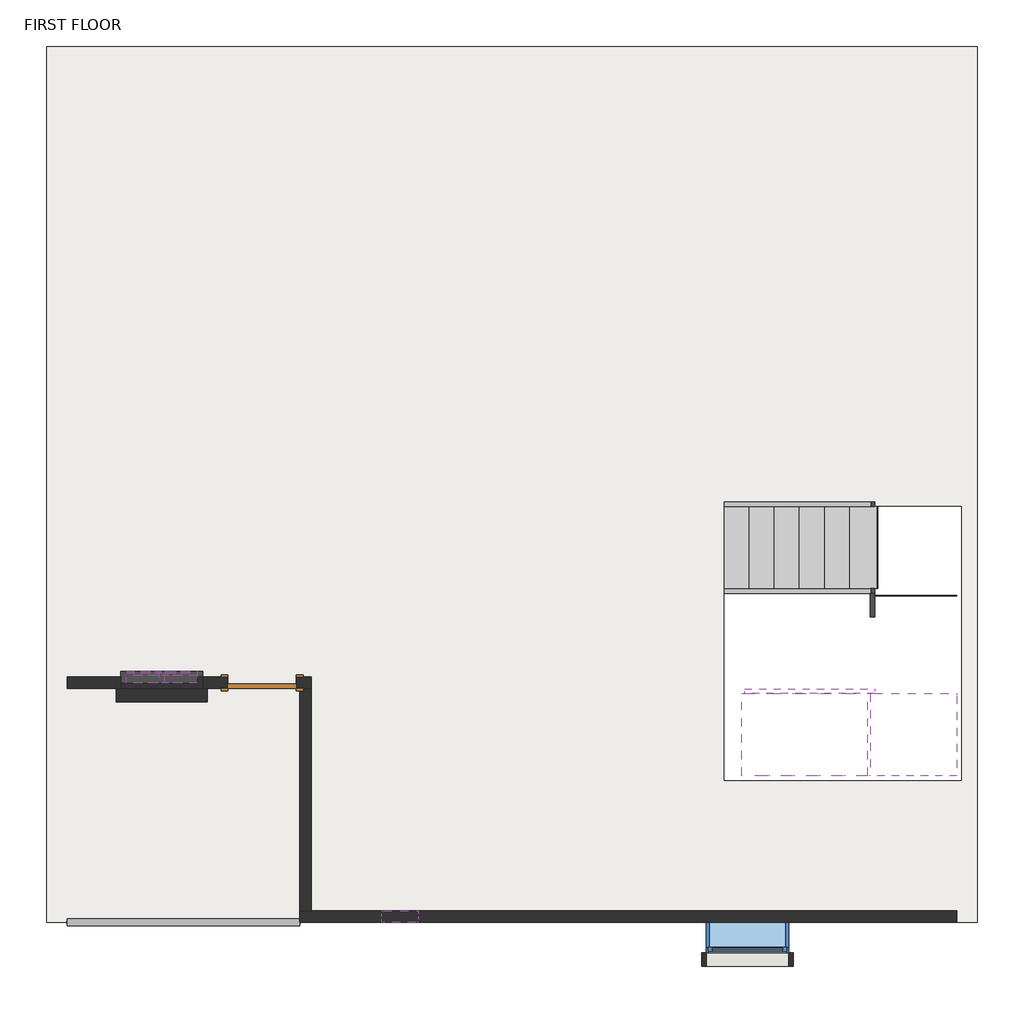
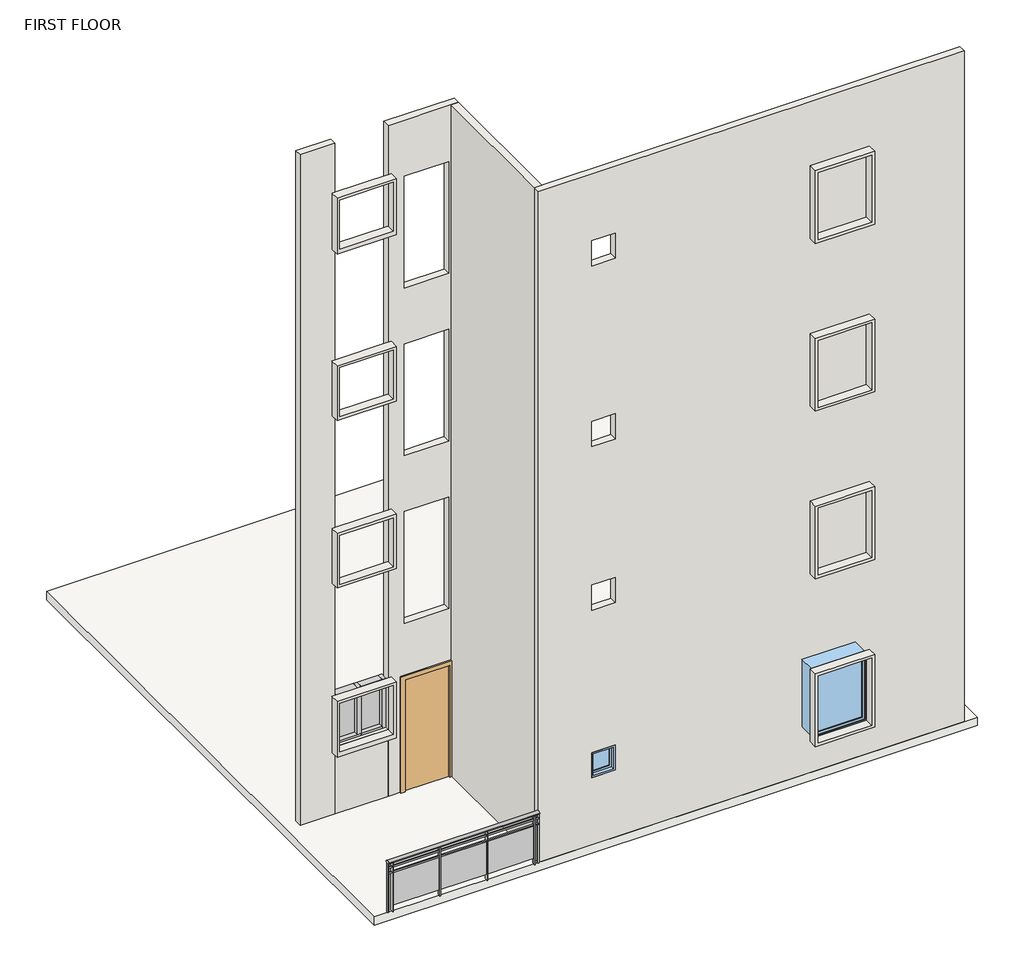
# One storey, incomplete: 15 members, 7 walls, 3 plates, 3 stair flights, 2 slabs, 2 windows, 1 door, 1 railing.
"""IFC4 building model written with IfcOpenShell, lengths in millimetres."""

from ifc_helpers import new_model, si_unit, point, frame, origin, place, context, project, spatial, polyline, ellipse_curve, trimmed, outline, extrude, faceted_brep, transform, mapped, element, save
from ifc_brep_helpers import plane_surface, extruded_surface, advanced_brep
from components import door_e00f436c, member_429f6687, member_d959a85f, member_843225dc, member_54f829b7, system_panel_glazed_1e360deb, system_panel_glazed_8fc33089, non_monolithic_landing_440175ab, stair_flight_60bc6d16, stair_flight_15cb6ebf, stair_flight_16b82674, walls_8_walls_8_31a24d2c, walls_9_walls_9_93cd2fbd, fixed_bw_be0fa6e9, fixed_ven_0bde2124

model = new_model("IFC4")

# Units and contexts
model_context = context("Model", 3, world=origin())
ifc_project = project(units=[si_unit("LENGTHUNIT", "METRE", prefix="MILLI")], contexts=[model_context])

# Site, building, storey
site = spatial("IfcSite", under=ifc_project)
building = spatial("IfcBuilding", under=site)
storey = spatial("IfcBuildingStorey", under=building, Name="FIRST FLOOR", Elevation=3048.0)

# Door
placement = place(None, origin())
door_shape = door_e00f436c(model_context)
element("IfcDoor", 1, ObjectType="Single-Flush : 36\" x 84\"", at=placement, inside=storey, context=model_context, shape_type="MappedRepresentation", body=[
    mapped(door_shape, transform((-4124.5569651, 3118.5055142, 3048.0), x_axis=(1.0, 0.0, 0.0), y_axis=(0.0, 1.0, 0.0), z_axis=(0.0, 0.0, 1.0))),
])

# Members
member_shape = member_429f6687(model_context)
element("IfcMember", 2, ObjectType="Rectangular Mullion : 2.5\" x 5\" rectangular", at=placement, inside=storey, context=model_context, shape_type="MappedRepresentation", body=[
    mapped(member_shape, transform((-4848.4569651, 3182.0055142, 5156.2), x_axis=(0.0, 0.0, 1.0), y_axis=(0.0, -1.0, 0.0), z_axis=(1.0, 0.0, 0.0))),
])
element("IfcMember", 3, ObjectType="Rectangular Mullion : 2.5\" x 5\" rectangular", at=placement, inside=storey, context=model_context, shape_type="MappedRepresentation", body=[
    mapped(member_shape, transform((-5635.8569651, 3182.0055142, 4237.4584417), x_axis=(0.0, 0.0, -1.0), y_axis=(0.0, -1.0, 0.0), z_axis=(-1.0, 0.0, 0.0))),
])
member_2_shape = member_d959a85f(model_context)
element("IfcMember", 4, ObjectType="Rectangular Mullion : 2.5\" x 5\" rectangular", at=placement, inside=storey, context=model_context, shape_type="MappedRepresentation", body=[
    mapped(member_2_shape, transform((-4784.9569651, 3182.0055142, 4237.4584417), x_axis=(1.0, 0.0, 0.0), y_axis=(0.0, -1.0, 0.0), z_axis=(0.0, 0.0, -1.0))),
])
element("IfcMember", 5, ObjectType="Rectangular Mullion : 2.5\" x 5\" rectangular", at=placement, inside=storey, context=model_context, shape_type="MappedRepresentation", body=[
    mapped(member_2_shape, transform((-4784.9569651, 3182.0055142, 4237.4584417), x_axis=(1.0, 0.0, 0.0), y_axis=(0.0, -1.0, 0.0), z_axis=(0.0, 0.0, -1.0))),
])
element("IfcMember", 6, ObjectType="Rectangular Mullion : 2.5\" x 5\" rectangular", at=placement, inside=storey, context=model_context, shape_type="MappedRepresentation", body=[
    mapped(member_2_shape, transform((-5699.3569651, 3182.0055142, 5156.2), x_axis=(-1.0, 0.0, 0.0), y_axis=(0.0, -1.0, 0.0), z_axis=(0.0, 0.0, 1.0))),
])
element("IfcMember", 7, ObjectType="Rectangular Mullion : 2.5\" x 5\" rectangular", at=placement, inside=storey, context=model_context, shape_type="MappedRepresentation", body=[
    mapped(member_2_shape, transform((-5699.3569651, 3182.0055142, 5156.2), x_axis=(-1.0, 0.0, 0.0), y_axis=(0.0, -1.0, 0.0), z_axis=(0.0, 0.0, 1.0))),
])
member_3_shape = member_843225dc(model_context)
element("IfcMember", 8, ObjectType="Rectangular Mullion : 2.5\" x 5\" rectangular", at=placement, inside=storey, context=model_context, shape_type="MappedRepresentation", body=[
    mapped(member_3_shape, transform((-4848.4569651, 3182.0055142, 5156.2), x_axis=(0.0, 0.0, 1.0), y_axis=(0.0, -1.0, 0.0), z_axis=(1.0, 0.0, 0.0))),
])
element("IfcMember", 9, ObjectType="Rectangular Mullion : 2.5\" x 5\" rectangular", at=placement, inside=storey, context=model_context, shape_type="MappedRepresentation", body=[
    mapped(member_3_shape, transform((-5273.9069651, 3182.0055142, 5156.2), x_axis=(0.0, 0.0, 1.0), y_axis=(0.0, -1.0, 0.0), z_axis=(1.0, 0.0, 0.0))),
])
element("IfcMember", 10, ObjectType="Rectangular Mullion : 2.5\" x 5\" rectangular", at=placement, inside=storey, context=model_context, shape_type="MappedRepresentation", body=[
    mapped(member_3_shape, transform((-5635.8569651, 3182.0055142, 4237.4584417), x_axis=(0.0, 0.0, -1.0), y_axis=(0.0, -1.0, 0.0), z_axis=(-1.0, 0.0, 0.0))),
])
element("IfcMember", 11, ObjectType="Rectangular Mullion : 2.5\" x 5\" rectangular", at=placement, inside=storey, context=model_context, shape_type="MappedRepresentation", body=[
    mapped(member_3_shape, transform((-5210.4069651, 3182.0055142, 4237.4584417), x_axis=(0.0, 0.0, -1.0), y_axis=(0.0, -1.0, 0.0), z_axis=(-1.0, 0.0, 0.0))),
])
member_4_shape = member_54f829b7(model_context)
element("IfcMember", 12, ObjectType="Rectangular Mullion : 2.5\" x 5\" rectangular", at=placement, inside=storey, context=model_context, shape_type="MappedRepresentation", body=[
    mapped(member_4_shape, transform((-5242.1569651, 3182.0055142, 4237.4584417), x_axis=(1.0, 0.0, 0.0), y_axis=(0.0, -1.0, 0.0), z_axis=(0.0, 0.0, -1.0))),
])
element("IfcMember", 13, ObjectType="Stringer - 2\" Width", at=placement, inside=storey, context=model_context, shape_type="SweptSolid", body=[
    extrude(outline(polyline([(3260.114512, 1018.9430349), (3048.0, 1018.9430349), (3048.0, 1257.0285467), (3919.7057504, 2695.3430349), (4276.114512, 2695.3430349), (3260.114512, 1018.9430349)])), frame((0.0, 5080.6555142, 0.0), z_axis=(0.0, 1.0, 0.0), x_axis=(0.0, 0.0, 1.0)), (0.0, 0.0, 1.0), 50.8),
])
element("IfcMember", 14, ObjectType="Stringer - 2\" Width", at=placement, inside=storey, context=model_context, shape_type="SweptSolid", body=[
    extrude(outline(polyline([(3260.114512, 1018.9430349), (3048.0, 1018.9430349), (3048.0, 1257.0285467), (3919.7057504, 2695.3430349), (4276.114512, 2695.3430349), (3260.114512, 1018.9430349)])), frame((0.0, 4115.4555142, 0.0), z_axis=(0.0, 1.0, 0.0), x_axis=(0.0, 0.0, 1.0)), (0.0, 0.0, 1.0), 50.8),
])
element("IfcMember", 15, ObjectType="Stringer - 2\" Width", at=placement, inside=storey, context=model_context, shape_type="SweptSolid", body=[
    extrude(outline(polyline([(4115.4555142, 4445.4478453), (4115.4555142, 4089.0390838), (3048.6555142, 4735.5845383), (3048.6555142, 5091.9932998), (4115.4555142, 4445.4478453)])), frame((2644.5430349, 0.0, 0.0), z_axis=(1.0, 0.0, 0.0), x_axis=(0.0, 1.0, 0.0)), (0.0, 0.0, 1.0), 50.8),
])
element("IfcMember", 16, ObjectType="Stringer - 2\" Width", at=placement, inside=storey, context=model_context, shape_type="SweptSolid", body=[
    extrude(outline(polyline([(4904.9178717, 2695.3430349), (5261.3266332, 2695.3430349), (6138.7811786, 1247.5430349), (5782.3724171, 1247.5430349), (4904.9178717, 2695.3430349)])), frame((0.0, 2997.8555142, 0.0), z_axis=(0.0, 1.0, 0.0), x_axis=(0.0, 0.0, 1.0)), (0.0, 0.0, 1.0), 50.8),
])

# Plates
system_panel_glazed_shape = system_panel_glazed_1e360deb(model_context)
element("IfcPlate", 17, ObjectType="System Panel : Glazed", at=placement, inside=storey, context=model_context, shape_type="MappedRepresentation", body=[
    mapped(system_panel_glazed_shape, transform((-5242.1569651, 3182.0055142, 4300.9584417), x_axis=(1.0, 0.0, 0.0), y_axis=(0.0, 1.0, 0.0), z_axis=(0.0, 0.0, 1.0))),
])
system_panel_glazed_2_shape = system_panel_glazed_8fc33089(model_context)
element("IfcPlate", 18, ObjectType="System Panel : Glazed", at=placement, inside=storey, context=model_context, shape_type="MappedRepresentation", body=[
    mapped(system_panel_glazed_2_shape, transform((-5454.8819651, 3182.0055142, 4300.9584417), x_axis=(1.0, 0.0, 0.0), y_axis=(0.0, 1.0, 0.0), z_axis=(0.0, 0.0, 1.0))),
])
element("IfcPlate", 19, ObjectType="System Panel : Glazed", at=placement, inside=storey, context=model_context, shape_type="MappedRepresentation", body=[
    mapped(system_panel_glazed_2_shape, transform((-5029.4319651, 3182.0055142, 4300.9584417), x_axis=(1.0, 0.0, 0.0), y_axis=(0.0, 1.0, 0.0), z_axis=(0.0, 0.0, 1.0))),
])

# Railing
element("IfcRailing", 20, ObjectType="Glass Panel - Bottom Fill", at=placement, inside=storey, context=model_context, shape_type="SolidModel", body=[
    advanced_brep(
    [(-6296.2569651, 489.6055142, 3962.4), (-6296.2569651, 413.4055142, 3962.4), (-3705.4569651, 489.6055142, 3962.4), (-3705.4569651, 413.4055142, 3962.4)],
    [
        (0, 1, ellipse_curve(frame((-6296.2569651, 451.5055142, 3962.4), z_axis=(-1.0, 0.0, 0.0), x_axis=(0.0, -1.0, 0.0)), 38.1, 28.575)),
        (1, 0, ellipse_curve(frame((-6296.2569651, 451.5055142, 3962.4), z_axis=(-1.0, 0.0, 0.0), x_axis=(0.0, -1.0, 0.0)), 38.1, 28.575)),
        (2, 3, ellipse_curve(frame((-3705.4569651, 451.5055142, 3962.4), z_axis=(1.0, 0.0, 0.0), x_axis=(0.0, -1.0, 0.0)), 38.1, 28.575)),
        (3, 2, ellipse_curve(frame((-3705.4569651, 451.5055142, 3962.4), z_axis=(1.0, 0.0, 0.0), x_axis=(0.0, -1.0, 0.0)), 38.1, 28.575)),
        (0, 2),
        (3, 1),
    ],
    [
        plane_surface(frame((-6296.2569651, 451.5055142, 3962.4), z_axis=(-1.0, 0.0, 0.0), x_axis=(0.0, 1.0, 0.0))),
        plane_surface(frame((-3705.4569651, 451.5055142, 3962.4), z_axis=(1.0, 0.0, 0.0), x_axis=(0.0, 1.0, 0.0))),
        extruded_surface(trimmed(ellipse_curve(frame((-3705.4569651, 451.5055142, 3962.4), z_axis=(-1.0, 0.0, 0.0), x_axis=(0.0, -1.0, 0.0)), 38.1, 28.575), [point((-3705.4569651, 489.6055142, 3962.4))], [point((-3705.4569651, 413.4055142, 3962.4))], True, "CARTESIAN"), (-2590.8, 0.0, 0.0), 2590.8),
        extruded_surface(trimmed(ellipse_curve(frame((-3705.4569651, 451.5055142, 3962.4), z_axis=(-1.0, 0.0, 0.0), x_axis=(0.0, -1.0, 0.0)), 38.1, 28.575), [point((-3705.4569651, 413.4055142, 3962.4))], [point((-3705.4569651, 489.6055142, 3962.4))], True, "CARTESIAN"), (-2590.8, 0.0, 0.0), 2590.8),
    ],
    [
        (0, [[1, 2]]),
        (1, [[3, 4]]),
        (2, [[-1, 5, -4, 6]]),
        (3, [[-2, -6, -3, -5]]),
    ],
),
    extrude(outline(polyline([(-6296.2569651, 438.8055142), (-6296.2569651, 464.2055142), (-3705.4569651, 464.2055142), (-3705.4569651, 438.8055142), (-6296.2569651, 438.8055142)])), frame((0.0, 0.0, 3848.1), z_axis=(0.0, 0.0, 1.0), x_axis=(1.0, 0.0, 0.0)), (0.0, 0.0, 1.0), 25.4),
    extrude(outline(polyline([(-6296.2569651, 438.8055142), (-6296.2569651, 464.2055142), (-3705.4569651, 464.2055142), (-3705.4569651, 438.8055142), (-6296.2569651, 438.8055142)])), frame((0.0, 0.0, 3746.5), z_axis=(0.0, 0.0, 1.0), x_axis=(1.0, 0.0, 0.0)), (0.0, 0.0, 1.0), 25.4),
    extrude(outline(polyline([(-3788.0069651, 426.1055142), (-3788.0069651, 476.9055142), (-3775.3069651, 476.9055142), (-3775.3069651, 426.1055142), (-3788.0069651, 426.1055142)])), frame((0.0, 0.0, 3048.0), z_axis=(0.0, 0.0, 1.0), x_axis=(1.0, 0.0, 0.0)), (0.0, 0.0, 1.0), 885.6788223),
    extrude(outline(polyline([(-4594.4569651, 458.0406712), (-3781.6569651, 458.0406712), (-3781.6569651, 451.6906712), (-4594.4569651, 451.6906712), (-4594.4569651, 458.0406712)])), frame((0.0, 0.0, 3149.6), z_axis=(0.0, 0.0, 1.0), x_axis=(1.0, 0.0, 0.0)), (0.0, 0.0, 1.0), 596.9),
    extrude(outline(polyline([(-4600.8069651, 426.1055142), (-4600.8069651, 476.9055142), (-4588.1069651, 476.9055142), (-4588.1069651, 426.1055142), (-4600.8069651, 426.1055142)])), frame((0.0, 0.0, 3048.0), z_axis=(0.0, 0.0, 1.0), x_axis=(1.0, 0.0, 0.0)), (0.0, 0.0, 1.0), 885.6788223),
    extrude(outline(polyline([(-5407.2569651, 458.0406712), (-4594.4569651, 458.0406712), (-4594.4569651, 451.6906712), (-5407.2569651, 451.6906712), (-5407.2569651, 458.0406712)])), frame((0.0, 0.0, 3149.6), z_axis=(0.0, 0.0, 1.0), x_axis=(1.0, 0.0, 0.0)), (0.0, 0.0, 1.0), 596.9),
    extrude(outline(polyline([(-5413.6069651, 426.1055142), (-5413.6069651, 476.9055142), (-5400.9069651, 476.9055142), (-5400.9069651, 426.1055142), (-5413.6069651, 426.1055142)])), frame((0.0, 0.0, 3048.0), z_axis=(0.0, 0.0, 1.0), x_axis=(1.0, 0.0, 0.0)), (0.0, 0.0, 1.0), 885.6788223),
    extrude(outline(polyline([(-6220.0569651, 458.0406712), (-5407.2569651, 458.0406712), (-5407.2569651, 451.6906712), (-6220.0569651, 451.6906712), (-6220.0569651, 458.0406712)])), frame((0.0, 0.0, 3149.6), z_axis=(0.0, 0.0, 1.0), x_axis=(1.0, 0.0, 0.0)), (0.0, 0.0, 1.0), 596.9),
    extrude(outline(polyline([(-6226.4069651, 426.1055142), (-6226.4069651, 476.9055142), (-6213.7069651, 476.9055142), (-6213.7069651, 426.1055142), (-6226.4069651, 426.1055142)])), frame((0.0, 0.0, 3048.0), z_axis=(0.0, 0.0, 1.0), x_axis=(1.0, 0.0, 0.0)), (0.0, 0.0, 1.0), 885.6788223),
    extrude(outline(polyline([(-3718.1569651, 441.9805142), (-3718.1569651, 461.0305142), (-3699.1069651, 461.0305142), (-3699.1069651, 441.9805142), (-3718.1569651, 441.9805142)])), frame((0.0, 0.0, 3048.0), z_axis=(0.0, 0.0, 1.0), x_axis=(1.0, 0.0, 0.0)), (0.0, 0.0, 1.0), 885.6788223),
    extrude(outline(polyline([(-6302.6069651, 441.9805142), (-6302.6069651, 461.0305142), (-6283.5569651, 461.0305142), (-6283.5569651, 441.9805142), (-6302.6069651, 441.9805142)])), frame((0.0, 0.0, 3048.0), z_axis=(0.0, 0.0, 1.0), x_axis=(1.0, 0.0, 0.0)), (0.0, 0.0, 1.0), 885.6788223),
])

# Slabs
element("IfcSlab", 21, ObjectType="Generic - 12\"", at=placement, inside=storey, context=model_context, shape_type="SweptSolid", body=[
    extrude(outline(polyline([(3838.3430349, 10205.1055142), (3838.3430349, 451.5055142), (-6524.8569651, 451.5055142), (-6524.8569651, 10205.1055142), (3838.3430349, 10205.1055142)]), holes=[polyline([(3660.5430349, 5080.6555142), (1018.9430349, 5080.6555142), (1018.9430349, 2032.6555142), (3660.5430349, 2032.6555142), (3660.5430349, 5080.6555142)])]), frame((0.0, 0.0, 2895.6), z_axis=(0.0, 0.0, 1.0), x_axis=(1.0, 0.0, 0.0)), (0.0, 0.0, 1.0), 152.4),
])
non_monolithic_landing_shape = non_monolithic_landing_440175ab(model_context)
element("IfcSlab", 22, ObjectType="Non-Monolithic Landing", at=placement, inside=storey, context=model_context, shape_type="MappedRepresentation", body=[
    mapped(non_monolithic_landing_shape, transform((0.0, 0.0, 0.0), x_axis=(1.0, 0.0, 0.0), y_axis=(0.0, 1.0, 0.0), z_axis=(0.0, 0.0, 1.0))),
])

# Stair flights
stair_flight_shape = stair_flight_60bc6d16(model_context)
element("IfcStairFlight", 23, ObjectType="2\" Tread 1\" Nosing 1/4\" Riser", at=placement, inside=storey, context=model_context, shape_type="MappedRepresentation", body=[
    mapped(stair_flight_shape, transform((0.0, 0.0, 0.0), x_axis=(1.0, 0.0, 0.0), y_axis=(0.0, 1.0, 0.0), z_axis=(0.0, 0.0, 1.0))),
])
stair_flight_2_shape = stair_flight_15cb6ebf(model_context)
element("IfcStairFlight", 24, ObjectType="2\" Tread 1\" Nosing 1/4\" Riser", at=placement, inside=storey, context=model_context, shape_type="MappedRepresentation", body=[
    mapped(stair_flight_2_shape, transform((0.0, 0.0, 0.0), x_axis=(1.0, 0.0, 0.0), y_axis=(0.0, 1.0, 0.0), z_axis=(0.0, 0.0, 1.0))),
])
stair_flight_3_shape = stair_flight_16b82674(model_context)
element("IfcStairFlight", 25, ObjectType="2\" Tread 1\" Nosing 1/4\" Riser", at=placement, inside=storey, context=model_context, shape_type="MappedRepresentation", body=[
    mapped(stair_flight_3_shape, transform((0.0, 0.0, 0.0), x_axis=(1.0, 0.0, 0.0), y_axis=(0.0, 1.0, 0.0), z_axis=(0.0, 0.0, 1.0))),
])

# Walls
element("IfcWall", 26, ObjectType="5\"", at=placement, inside=storey, context=model_context, shape_type="Brep", body=[
    faceted_brep([(3609.7430349, 578.5055142, 3048.0), (-3578.4569651, 578.5055142, 3048.0), (-3705.4569651, 578.5055142, 3048.0), (-3705.4569651, 578.5055142, 15240.0), (-3578.4569651, 578.5055142, 15240.0), (3609.7430349, 578.5055142, 15240.0), (-2384.6569651, 578.5055142, 4724.6018374), (-2791.0569651, 578.5055142, 4724.6018374), (-2791.0569651, 578.5055142, 4267.4018374), (-2384.6569651, 578.5055142, 4267.4018374), (-2384.6569651, 578.5055142, 7768.6646104), (-2791.0569651, 578.5055142, 7768.6646104), (-2791.0569651, 578.5055142, 7311.4646104), (-2384.6569651, 578.5055142, 7311.4646104), (-2384.6569651, 578.5055142, 10741.382033), (-2791.0569651, 578.5055142, 10741.382033), (-2791.0569651, 578.5055142, 10284.182033), (-2384.6569651, 578.5055142, 10284.182033), (-2384.6569651, 578.5055142, 14028.295937), (-2791.0569651, 578.5055142, 14028.295937), (-2791.0569651, 578.5055142, 13571.095937), (-2384.6569651, 578.5055142, 13571.095937), (3609.7430349, 451.5055142, 3048.0), (3609.7430349, 451.5055142, 15240.0), (-3705.4569651, 451.5055142, 15240.0), (-3705.4569651, 451.5055142, 3048.0), (-2384.6569651, 451.5055142, 4724.6018374), (-2384.6569651, 451.5055142, 4267.4018374), (-2791.0569651, 451.5055142, 4267.4018374), (-2791.0569651, 451.5055142, 4724.6018374), (-2384.6569651, 451.5055142, 7768.6646104), (-2384.6569651, 451.5055142, 7311.4646104), (-2791.0569651, 451.5055142, 7311.4646104), (-2791.0569651, 451.5055142, 7768.6646104), (-2384.6569651, 451.5055142, 10741.382033), (-2384.6569651, 451.5055142, 10284.182033), (-2791.0569651, 451.5055142, 10284.182033), (-2791.0569651, 451.5055142, 10741.382033), (-2384.6569651, 451.5055142, 14028.295937), (-2384.6569651, 451.5055142, 13571.095937), (-2791.0569651, 451.5055142, 13571.095937), (-2791.0569651, 451.5055142, 14028.295937)], [[[0, 1, 2, 3, 4, 5], [6, 7, 8, 9], [10, 11, 12, 13], [14, 15, 16, 17], [18, 19, 20, 21]], [[22, 23, 24, 25], [26, 27, 28, 29], [30, 31, 32, 33], [34, 35, 36, 37], [38, 39, 40, 41]], [[2, 1, 0, 22, 25]], [[5, 4, 3, 24, 23]], [[0, 5, 23, 22]], [[3, 2, 25, 24]], [[27, 26, 6, 9]], [[28, 27, 9, 8]], [[29, 28, 8, 7]], [[26, 29, 7, 6]], [[31, 30, 10, 13]], [[32, 31, 13, 12]], [[33, 32, 12, 11]], [[30, 33, 11, 10]], [[35, 34, 14, 17]], [[36, 35, 17, 16]], [[37, 36, 16, 15]], [[34, 37, 15, 14]], [[39, 38, 18, 21]], [[40, 39, 21, 20]], [[41, 40, 20, 19]], [[38, 41, 19, 18]]]),
])
element("IfcWall", 27, ObjectType="5\"", at=placement, inside=storey, context=model_context, shape_type="Brep", body=[
    faceted_brep([(-6296.2569651, 3055.0055142, 3048.0), (-5699.3569651, 3055.0055142, 3048.0), (-5699.3569651, 3055.0055142, 5156.2), (-5699.3569651, 3055.0055142, 7315.2), (-5699.3569651, 3055.0055142, 8204.2), (-5699.3569651, 3055.0055142, 10363.2), (-5699.3569651, 3055.0055142, 11252.2), (-5699.3569651, 3055.0055142, 13411.2), (-5699.3569651, 3055.0055142, 14300.2), (-5699.3569651, 3055.0055142, 15240.0), (-6296.2569651, 3055.0055142, 15240.0), (-6296.2569651, 3182.0055142, 3048.0), (-6296.2569651, 3182.0055142, 15240.0), (-5699.3569651, 3182.0055142, 15240.0), (-5699.3569651, 3182.0055142, 14300.2), (-5699.3569651, 3182.0055142, 13411.2), (-5699.3569651, 3182.0055142, 11252.2), (-5699.3569651, 3182.0055142, 10363.2), (-5699.3569651, 3182.0055142, 8204.2), (-5699.3569651, 3182.0055142, 7315.2), (-5699.3569651, 3182.0055142, 5156.2), (-5699.3569651, 3182.0055142, 4267.2), (-5699.3569651, 3182.0055142, 3048.0)], [[[0, 1, 2, 3, 4, 5, 6, 7, 8, 9, 10]], [[11, 12, 13, 14, 15, 16, 17, 18, 19, 20, 21, 22]], [[1, 0, 11, 22]], [[10, 9, 13, 12]], [[0, 10, 12, 11]], [[1, 22, 21, 20, 19, 18, 17, 16, 15, 14, 13, 9, 8, 7, 6, 5, 4, 3, 2]]]),
])
element("IfcWall", 28, ObjectType="5\"", at=placement, inside=storey, context=model_context, shape_type="SweptSolid", body=[
    extrude(outline(polyline([(-3705.4569651, 578.5055142), (-3705.4569651, 3055.0055142), (-3578.4569651, 3055.0055142), (-3578.4569651, 578.5055142), (-3705.4569651, 578.5055142)])), frame((0.0, 0.0, 3048.0), z_axis=(0.0, 0.0, 1.0), x_axis=(1.0, 0.0, 0.0)), (0.0, 0.0, 1.0), 12192.0),
])
element("IfcWall", 29, ObjectType="5\"", at=placement, inside=storey, context=model_context, shape_type="Brep", body=[
    faceted_brep([(-3743.5569651, 3055.0055142, 5080.0), (-3743.5569651, 3055.0055142, 3048.0), (-3705.4569651, 3055.0055142, 3048.0), (-3578.4569651, 3055.0055142, 3048.0), (-3578.4569651, 3055.0055142, 15240.0), (-3705.4569651, 3055.0055142, 15240.0), (-4784.9569651, 3055.0055142, 15240.0), (-4784.9569651, 3055.0055142, 14300.2), (-4784.9569651, 3055.0055142, 13411.2), (-4784.9569651, 3055.0055142, 11252.2), (-4784.9569651, 3055.0055142, 10363.2), (-4784.9569651, 3055.0055142, 8204.2), (-4784.9569651, 3055.0055142, 7315.2), (-4784.9569651, 3055.0055142, 5156.2), (-4784.9569651, 3055.0055142, 4267.2), (-4784.9569651, 3055.0055142, 3048.0), (-4505.5569651, 3055.0055142, 3048.0), (-4505.5569651, 3055.0055142, 5080.0), (-4505.5569651, 3055.0055142, 12192.0), (-4505.5569651, 3055.0055142, 14224.0), (-3743.5569651, 3055.0055142, 14224.0), (-3743.5569651, 3055.0055142, 12192.0), (-4505.5569651, 3055.0055142, 6096.0), (-4505.5569651, 3055.0055142, 8128.0), (-3743.5569651, 3055.0055142, 8128.0), (-3743.5569651, 3055.0055142, 6096.0), (-4505.5569651, 3055.0055142, 9144.0), (-4505.5569651, 3055.0055142, 11176.0), (-3743.5569651, 3055.0055142, 11176.0), (-3743.5569651, 3055.0055142, 9144.0), (-3578.4569651, 3182.0055142, 3048.0), (-3743.5569651, 3182.0055142, 3048.0), (-3743.5569651, 3182.0055142, 5080.0), (-4505.5569651, 3182.0055142, 5080.0), (-4505.5569651, 3182.0055142, 3048.0), (-4784.9569651, 3182.0055142, 3048.0), (-4784.9569651, 3182.0055142, 4267.2), (-4784.9569651, 3182.0055142, 5156.2), (-4784.9569651, 3182.0055142, 7315.2), (-4784.9569651, 3182.0055142, 8204.2), (-4784.9569651, 3182.0055142, 10363.2), (-4784.9569651, 3182.0055142, 11252.2), (-4784.9569651, 3182.0055142, 13411.2), (-4784.9569651, 3182.0055142, 14300.2), (-4784.9569651, 3182.0055142, 15240.0), (-3578.4569651, 3182.0055142, 15240.0), (-4505.5569651, 3182.0055142, 12192.0), (-3743.5569651, 3182.0055142, 12192.0), (-3743.5569651, 3182.0055142, 14224.0), (-4505.5569651, 3182.0055142, 14224.0), (-4505.5569651, 3182.0055142, 6096.0), (-3743.5569651, 3182.0055142, 6096.0), (-3743.5569651, 3182.0055142, 8128.0), (-4505.5569651, 3182.0055142, 8128.0), (-4505.5569651, 3182.0055142, 9144.0), (-3743.5569651, 3182.0055142, 9144.0), (-3743.5569651, 3182.0055142, 11176.0), (-4505.5569651, 3182.0055142, 11176.0)], [[[0, 1, 2, 3, 4, 5, 6, 7, 8, 9, 10, 11, 12, 13, 14, 15, 16, 17], [18, 19, 20, 21], [22, 23, 24, 25], [26, 27, 28, 29]], [[30, 31, 32, 33, 34, 35, 36, 37, 38, 39, 40, 41, 42, 43, 44, 45], [46, 47, 48, 49], [50, 51, 52, 53], [54, 55, 56, 57]], [[16, 15, 35, 34]], [[3, 2, 1, 31, 30]], [[6, 5, 4, 45, 44]], [[4, 3, 30, 45]], [[34, 33, 17, 16]], [[33, 32, 0, 17]], [[32, 31, 1, 0]], [[46, 49, 19, 18]], [[49, 48, 20, 19]], [[48, 47, 21, 20]], [[47, 46, 18, 21]], [[50, 53, 23, 22]], [[53, 52, 24, 23]], [[52, 51, 25, 24]], [[51, 50, 22, 25]], [[54, 57, 27, 26]], [[57, 56, 28, 27]], [[56, 55, 29, 28]], [[55, 54, 26, 29]], [[6, 44, 43, 42, 41, 40, 39, 38, 37, 36, 35, 15, 14, 13, 12, 11, 10, 9, 8, 7]]]),
])
element("IfcWall", 30, ObjectType="5\"", at=placement, inside=storey, context=model_context, shape_type="SweptSolid", body=[
    extrude(outline(polyline([(-4784.9569651, 3055.0055142), (-5699.3569651, 3055.0055142), (-5699.3569651, 3182.0055142), (-4784.9569651, 3182.0055142), (-4784.9569651, 3055.0055142)])), frame((0.0, 0.0, 3048.0), z_axis=(0.0, 0.0, 1.0), x_axis=(1.0, 0.0, 0.0)), (0.0, 0.0, 1.0), 1219.2),
])
walls_8_walls_8_shape = walls_8_walls_8_31a24d2c(model_context)
element("IfcWall", 31, ObjectType="Walls 8 : Walls 8", at=placement, inside=storey, context=model_context, shape_type="MappedRepresentation", body=[
    mapped(walls_8_walls_8_shape, transform((0.0, 0.0, 0.0), x_axis=(1.0, 0.0, 0.0), y_axis=(0.0, 1.0, 0.0), z_axis=(0.0, 0.0, 1.0))),
])
walls_9_walls_9_shape = walls_9_walls_9_93cd2fbd(model_context)
element("IfcWall", 32, ObjectType="Walls 9 : Walls 9", at=placement, inside=storey, context=model_context, shape_type="MappedRepresentation", body=[
    mapped(walls_9_walls_9_shape, transform((0.0, 0.0, 0.0), x_axis=(1.0, 0.0, 0.0), y_axis=(0.0, 1.0, 0.0), z_axis=(0.0, 0.0, 1.0))),
])

# Windows
fixed_bw_shape = fixed_bw_be0fa6e9(model_context)
element("IfcWindow", 33, ObjectType="Fixed : BW", at=placement, inside=storey, context=model_context, shape_type="MappedRepresentation", body=[
    mapped(fixed_bw_shape, transform((1239.8073388, 281.3921573, 3022.6), x_axis=(-1.0, 0.0, 0.0), y_axis=(0.0, -1.0, 0.0), z_axis=(0.0, 0.0, 1.0))),
])
fixed_ven_shape = fixed_ven_0bde2124(model_context)
element("IfcWindow", 34, ObjectType="Fixed : VEN", at=placement, inside=storey, context=model_context, shape_type="MappedRepresentation", body=[
    mapped(fixed_ven_shape, transform((-2549.7569651, 515.0055142, 3353.0018374), x_axis=(1.0, 0.0, 0.0), y_axis=(0.0, 1.0, 0.0), z_axis=(0.0, 0.0, 1.0))),
])

save(model, "model.ifc")

# Revit data of these elements
# Type "Single-Flush : 36\" x 84\""
#   Type Mark = "1"
#   Construction Type Id = "MDOOR"
#   Assembly Code = "C1020"
#   Analytic Construction = "Metal"
#   Thickness = 0' - 2"
#   Heat Transfer Coefficient (U) = 0.651978 BTU/(h·ft²·°F)
#   Height = 6' - 8"
#   Trim Projection Ext = 0' - 1"
#   Trim Projection Int = 0' - 1"
#   Trim Width = 0' - 3"
#   Width = 2' - 6"
#   Define Thermal Properties by = 1
#   Define Thermal Properties by = 1
#   Door Material = Door - Panel
#   Frame Material = Door - Frame
#   Visual Light Transmittance = 0
#   Solar Heat Gain Coefficient = 0
#   Function = (empty or 0)
#   Wall Closure = (empty or 0)
# Type "Rectangular Mullion : 2.5\" x 5\" rectangular"
#   built-in parameter 1007304 = 0.416667 (stored number, unit not read)
#   built-in parameter 1007301 = 0.104167 (stored number, unit not read)
#   built-in parameter 1007300 = 0.104167 (stored number, unit not read)
# Type "System Panel : Glazed"
#   Construction Type Id = "GSP4R"
#   Analytic Construction = "1/8 in Pilkington single glazing"
#   Visual Light Transmittance = 0.9
#   Solar Heat Gain Coefficient = 0.86
#   Heat Transfer Coefficient (U) = 1.18115 BTU/(h·ft²·°F)
#   Define Thermal Properties by = 1
# Type "Glass Panel - Bottom Fill"
#   Assembly Code = "C2010400"
#   built-in parameter 1008612 = 0.0416667 (stored number, unit not read)
#   built-in parameter 1008611 = 0.0416667 (stored number, unit not read)
#   built-in parameter 1008609 = 0.333333 (stored number, unit not read)
#   built-in parameter 1008604 = 0.166667 (stored number, unit not read)
#   built-in parameter 1008603 = 0.166667 (stored number, unit not read)
#   Railing Height = 3' - 0"
#   built-in parameter 1008630 = 2
#   built-in parameter 1008610 = 2
#   built-in parameter 1008618 = Baluster - Square : 3/4"
# Type "Generic - 12\""
#   Assembly Code = "B1010"
#   Function = 0
#   Layers, outside or top first: 0' - 6" no material (function 1)
# Type "5\""
#   Assembly Code = "B2010"
#   Layers, outside or top first: 0' - 5" "Concrete Masonry Units" (function 1)
# Type "Fixed : BW"
#   Type Mark = "18"
#   Construction Type Id = "GSP4R"
#   Assembly Code = "B2020100"
#   Analytic Construction = "1/8 in Pilkington single glazing"
#   Visual Light Transmittance = 0.9
#   Solar Heat Gain Coefficient = 0.78
#   Heat Transfer Coefficient (U) = 0.6496 BTU/(h·ft²·°F)
#   Height = 4' - 0"
#   Default Sill Height = 3' - 0"
#   Width = 3' - 0"
#   Window Inset = 0' - 0 3/4"
#   Define Thermal Properties by = 1
#   Glass Pane Material = Glass
#   Sash Material = Sash
#   Wall Closure = (empty or 0)
# Type "Fixed : VEN"
#   Type Mark = "19"
#   Construction Type Id = "GSP4R"
#   Assembly Code = "B2020100"
#   Analytic Construction = "1/8 in Pilkington single glazing"
#   Visual Light Transmittance = 0.9
#   Solar Heat Gain Coefficient = 0.78
#   Heat Transfer Coefficient (U) = 0.6496 BTU/(h·ft²·°F)
#   Height = 1' - 6"
#   Default Sill Height = 3' - 0"
#   Width = 1' - 4"
#   Window Inset = 0' - 0 3/4"
#   Define Thermal Properties by = 1
#   Glass Pane Material = Glass
#   Sash Material = Sash
#   Wall Closure = (empty or 0)
# Element 1 (IfcDoor, "Single-Flush : 36\" x 84\"")
#   Phase Created = New Construction
#   Materials on its faces: "Door - Frame", "Door - Panel"
# Elements 2, 3, 4, 5, 6, 7, 8, 9, 10, 11, 12 (IfcMember, "Rectangular Mullion : 2.5\" x 5\" rectangular")
#   Phase Created = New Construction
#   Materials on its faces: "Aluminum"
# Elements 13, 14, 15, 16 (IfcMember, "Stringer - 2\" Width")
#   Phase Created = New Construction
# Elements 17, 18, 19 (IfcPlate, "System Panel : Glazed")
#   Phase Created = New Construction
#   Materials on its faces: "Glass"
# Element 20 (IfcRailing, "Glass Panel - Bottom Fill")
#   Phase Created = New Construction
#   Materials on its faces: "Glass", "1 wall white"
# Element 21 (IfcSlab, "Generic - 12\"")
#   Height Offset From Level = 0' - 0"
#   Phase Created = New Construction
#   Materials on its faces: "Default Floor", "1 wall white"
# Element 22 (IfcSlab, "Non-Monolithic Landing")
#   Phase Created = New Construction
# Elements 23, 24, 25 (IfcStairFlight, "2\" Tread 1\" Nosing 1/4\" Riser")
#   Phase Created = New Construction
# Element 26 (IfcWall, "5\"")
#   Top Offset = 0' - 0"
#   Base Offset = 0' - 0"
#   Unconnected Height = 40' - 0"
#   wall height = 40' - 0"
#   Phase Created = New Construction
#   Base Constraint = FIRST FLOOR
#   Materials on its faces: "Concrete Masonry Units", "1 wall brown", "1 wall white"
# Elements 27, 28, 29 (IfcWall, "5\"")
#   Top Offset = 0' - 0"
#   Base Offset = 0' - 0"
#   Unconnected Height = 40' - 0"
#   wall height = 40' - 0"
#   Phase Created = New Construction
#   Base Constraint = FIRST FLOOR
#   Materials on its faces: "Concrete Masonry Units", "1 wall white"
# Element 30 (IfcWall, "5\"")
#   Top Offset = 0' - 0"
#   Base Offset = 0' - 0"
#   Unconnected Height = 4' - 0"
#   wall height = 4' - 0"
#   Phase Created = New Construction
#   Base Constraint = FIRST FLOOR
#   Materials on its faces: "Concrete Masonry Units", "1 wall white"
# Element 31 (IfcWall, "Walls 8 : Walls 8")
#   Phase Created = New Construction
#   Materials on its faces: "1 wall white", "Default Wall"
# Element 32 (IfcWall, "Walls 9 : Walls 9")
#   Phase Created = New Construction
#   Materials on its faces: "Default Wall"
# Element 33 (IfcWindow, "Fixed : BW")
#   Mark = "6"
#   Phase Created = New Construction
#   Materials on its faces: "Sash", "Glass"
# Element 34 (IfcWindow, "Fixed : VEN")
#   Mark = "10"
#   Phase Created = New Construction
#   Materials on its faces: "Sash", "Glass"
# Materials
#   "Door - Panel": class "Wood", colour RGB 210 159 95, transparency 0, Cost = 0
#   "Door - Frame": colour RGB 118 70 51, transparency 0, Cost = 0
#   "Concrete Masonry Units": class "Masonry", colour RGB 227 227 227, transparency 0, Description = "Concrete masonry units", Cost = 0
#   "Glass": class "Glass", colour RGB 0 128 192, transparency 0.75, Description = "Soda Lime Glass", Cost = 0
#   "Sash": class "Wood", colour RGB 224 178 126, transparency 0, Cost = 0
#   "Aluminum": class "Metal", colour RGB 247 247 247, transparency 0, Description = "Aluminum 6061", Cost = 0
#   "1 wall white": class "Generic", colour RGB 244 245 241, transparency 0, Cost = 0
#   "Default Floor": colour RGB 128 128 128, transparency 0, Cost = 0
#   "1 wall brown": class "Generic", colour RGB 61 46 37, transparency 0, Cost = 0
#   "Default Wall": colour RGB 128 128 128, transparency 0, Cost = 0
